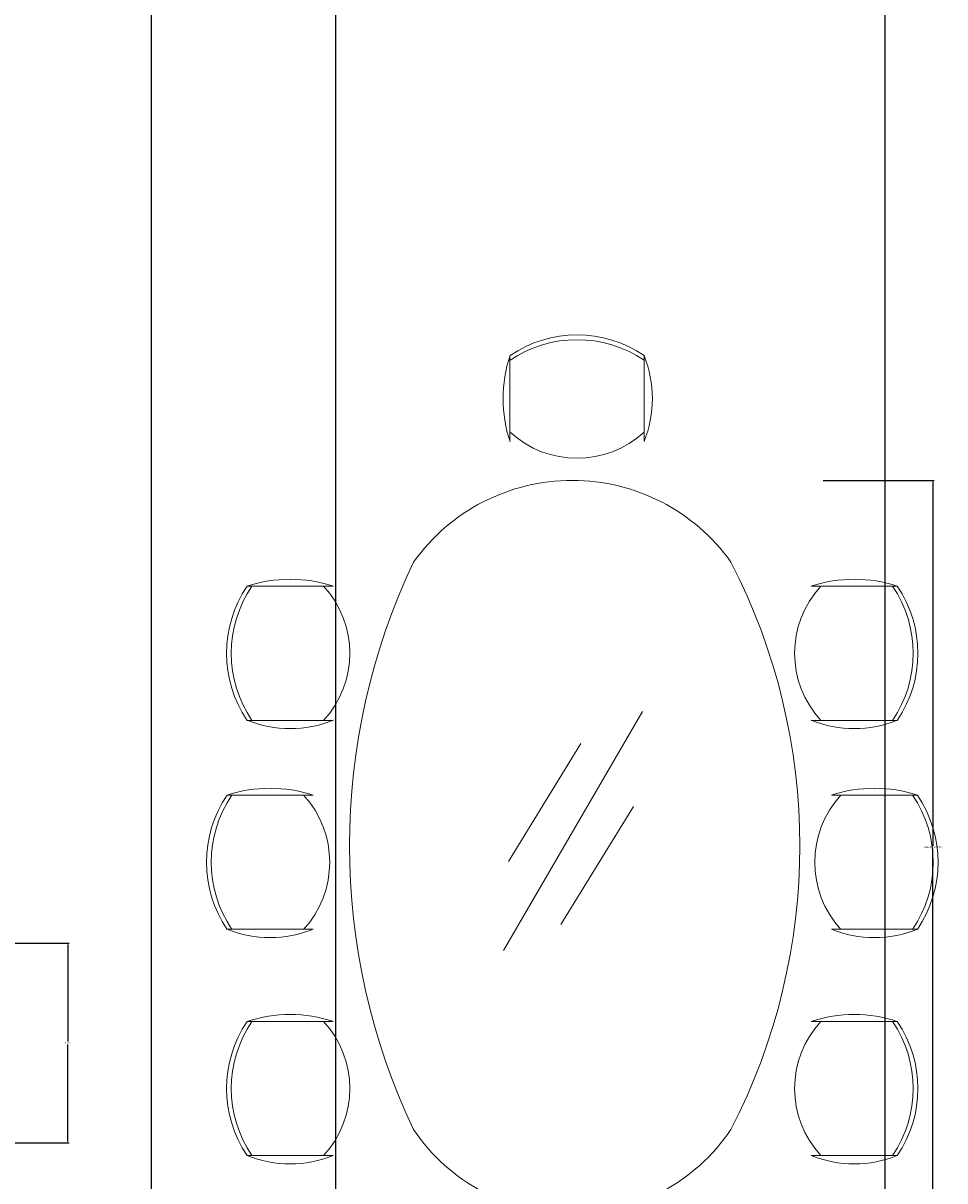
# Model space of a CAD drawing. Units: inches. Extents: x -61 to 1599, y -1316 to 257.
# Tile 125 of 204: x 236 to 356, y -166 to -16. Entities that reach past the tile are written whole.
import ezdxf

# ---------------------------------------------------------------- set-up
doc = ezdxf.new("R2010")
doc.units = ezdxf.units.IN
doc.header["$MEASUREMENT"] = 0
doc.layers.add('A-ANNO-DIMS', color=2, linetype='Continuous', lineweight=18)
doc.layers.add('FURNITURE', color=83, linetype='Continuous', lineweight=18)
doc.styles.get("Standard").update_dxf_attribs({"font": 'arial.ttf'})
doc.dimstyles.get("Standard").update_dxf_attribs({"dimtxt": 0.18, "dimasz": 0.18, "dimexe": 0.18, "dimexo": 0.0625, "dimgap": 0.09, "dimtad": 0, "dimtih": 1, "dimtoh": 1, "dimdec": 0, "dimzin": 0, "dimdsep": 46, "dimlunit": 3, "dimtxsty": 'Standard', "dimcen": 0.09, "dimadec": 0, "dimazin": 0, "dimtfac": 1, "dimtdec": 0, "dimtofl": 0, "dimtmove": 0, "dimatfit": 3, "dimfxl": 1, "dimtolj": 1, "dimtzin": 0, "dimarcsym": 0})

# ---------------------------------------------------------------- blocks, each defined once
blk = doc.blocks.new('DINING-TABLE-OVAL')
for p, q in [((20.06, 34.26), (38.12, 65.35)), ((20.69, 45.86), (30.12, 61.18)), ((27.51, 37.68), (36.94, 53.01))]:
    blk.add_line(p, q)
for centre, radius, start, end in [((28.99, 70.07), 25.36, 35.5172, 144.4828), ((85.79, 47.89), 85.79, 154.5151, 205.4849), ((-21.85, 47.89), 80.45, 332.689, 27.311), ((28.99, 24.89), 24.89, 213.9753, 326.0247)]:
    blk.add_arc(centre, radius, start, end)
blk = doc.blocks.new('DINING-CHAIR')
for p, q in [((0.9, 2.16), (0.9, 13.35)), ((18.35, 2.16), (18.35, 13.35))]:
    blk.add_line(p, q)
for centre, radius, start, end in [((9.63, 0.52), 15.52, 55.8098, 124.1902), ((9.63, -0.1), 15.52, 55.8098, 124.1902), ((17.78, 7.76), 17.78, 161.6455, 198.3545), ((4.51, 7.76), 14.92, 337.9646, 22.0354), ((9.63, 12.87), 12.87, 227.332, 312.668)]:
    blk.add_arc(centre, radius, start, end)
blk = doc.blocks.new('*D666')
at = {"layer": 'A-ANNO-DIMS', "color": 0, "lineweight": -2, "transparency": 16777216}
for p, q in [((340.28, -75.2), (354.71, -75.2)), ((354.53, -75.38), (354.53, -122.73)), ((354.53, -170.45), (354.53, -123.09)), ((340.28, -170.63), (354.71, -170.63))]:
    blk.add_line(p, q, dxfattribs=at)
at = {"layer": 'A-ANNO-DIMS', "color": 0, "transparency": 16777216}
for points in [[(354.5, -75.38), (354.56, -75.38), (354.53, -75.2)], [(354.5, -170.45), (354.56, -170.45), (354.53, -170.63)]]:
    blk.add_solid(points, dxfattribs=at)
at = {"layer": 'DEFPOINTS', "color": 0, "transparency": 16777216}
for p in [(340.22, -75.2), (354.53, -75.2), (340.22, -170.63)]:
    blk.add_point(p, dxfattribs=at)
at = {"layer": 'A-ANNO-DIMS', "color": 0, "transparency": 16777216, "insert": (354.53, -122.91), "char_height": 0.18, "attachment_point": 5}
blk.add_mtext('\\A1;DINING TABLE 95 TYP.', dxfattribs=at)
blk = doc.blocks.new('*D671')
at = {"layer": 'A-ANNO-DIMS', "color": 0, "lineweight": -2, "transparency": 16777216}
for p, q in [((229.44, -135.38), (242.15, -135.38)), ((241.97, -135.56), (241.97, -148.2)), ((241.97, -161.2), (241.97, -148.56)), ((229.44, -161.38), (242.15, -161.38))]:
    blk.add_line(p, q, dxfattribs=at)
at = {"layer": 'A-ANNO-DIMS', "color": 0, "transparency": 16777216}
for points in [[(241.94, -135.56), (242, -135.56), (241.97, -135.38)], [(241.94, -161.2), (242, -161.2), (241.97, -161.38)]]:
    blk.add_solid(points, dxfattribs=at)
at = {"layer": 'DEFPOINTS', "color": 0, "transparency": 16777216}
for p in [(229.37, -135.38), (241.97, -135.38), (229.37, -161.38)]:
    blk.add_point(p, dxfattribs=at)
at = {"layer": 'A-ANNO-DIMS', "color": 0, "transparency": 16777216, "insert": (241.97, -148.38), "char_height": 0.18, "attachment_point": 5}
blk.add_mtext('\\A1;26 TYP.', dxfattribs=at)
blk = doc.blocks.new('*D687')
at = {"layer": 'A-ANNO-DIMS', "color": 0, "lineweight": -2, "transparency": 16777216}
for p, q in [((289.42, 181.68), (-61.08, 181.68)), ((-60.9, 181.5), (-60.9, -528.95)), ((-60.9, -1239.76), (-60.9, -529.32)), ((319.64, -1239.94), (-61.08, -1239.94))]:
    blk.add_line(p, q, dxfattribs=at)
at = {"layer": 'A-ANNO-DIMS', "color": 0, "transparency": 16777216}
for points in [[(-60.93, 181.5), (-60.87, 181.5), (-60.9, 181.68)], [(-60.93, -1239.76), (-60.87, -1239.76), (-60.9, -1239.94)]]:
    blk.add_solid(points, dxfattribs=at)
at = {"layer": 'DEFPOINTS', "color": 0, "transparency": 16777216}
for p in [(289.48, 181.68), (-60.9, -1239.94), (319.7, -1239.94)]:
    blk.add_point(p, dxfattribs=at)
at = {"layer": 'A-ANNO-DIMS', "color": 0, "transparency": 16777216, "insert": (-60.9, -529.13), "char_height": 0.18, "attachment_point": 5}
blk.add_mtext('\\A1;1421.6', dxfattribs=at)
blk = doc.blocks.new('*D701')
at = {"layer": 'A-ANNO-DIMS', "color": 0, "lineweight": -2, "transparency": 16777216}
for p, q in [((215.75, -616.88), (215.75, 257.46)), ((215.93, 257.28), (233.92, 257.28)), ((252.7, 257.28), (234.71, 257.28)), ((252.88, -616.88), (252.88, 257.46))]:
    blk.add_line(p, q, dxfattribs=at)
at = {"layer": 'A-ANNO-DIMS', "color": 0, "transparency": 16777216}
for points in [[(215.93, 257.31), (215.93, 257.25), (215.75, 257.28)], [(252.7, 257.31), (252.7, 257.25), (252.88, 257.28)]]:
    blk.add_solid(points, dxfattribs=at)
at = {"layer": 'DEFPOINTS', "color": 0, "transparency": 16777216}
for p in [(252.88, 257.28), (215.75, -616.94), (252.88, -616.94)]:
    blk.add_point(p, dxfattribs=at)
at = {"layer": 'A-ANNO-DIMS', "color": 0, "transparency": 16777216, "insert": (234.32, 257.28), "char_height": 0.18, "attachment_point": 5}
blk.add_mtext('\\A1;37.13', dxfattribs=at)
blk = doc.blocks.new('*D702')
at = {"layer": 'A-ANNO-DIMS', "color": 0, "lineweight": -2, "transparency": 16777216}
for p, q in [((276.88, -616.88), (276.88, 257.46)), ((277.06, 257.28), (312.21, 257.28)), ((348.14, 257.28), (312.99, 257.28)), ((348.32, -616.88), (348.32, 257.46))]:
    blk.add_line(p, q, dxfattribs=at)
at = {"layer": 'A-ANNO-DIMS', "color": 0, "transparency": 16777216}
for points in [[(277.06, 257.31), (277.06, 257.25), (276.88, 257.28)], [(348.14, 257.31), (348.14, 257.25), (348.32, 257.28)]]:
    blk.add_solid(points, dxfattribs=at)
at = {"layer": 'DEFPOINTS', "color": 0, "transparency": 16777216}
for p in [(348.32, 257.28), (276.88, -616.94), (348.32, -616.94)]:
    blk.add_point(p, dxfattribs=at)
at = {"layer": 'A-ANNO-DIMS', "color": 0, "transparency": 16777216, "insert": (312.6, 257.28), "char_height": 0.18, "attachment_point": 5}
blk.add_mtext('\\A1;71.44', dxfattribs=at)

msp = doc.modelspace()

# ---------------------------------------------------------------- block references
at = {"layer": 'FURNITURE'}
for name, p in [('DINING-CHAIR', (298.622, -72.324)), ('DINING-TABLE-OVAL', (278.634, -170.626))]:
    msp.add_blockref(name, p, dxfattribs=at)
at = {"layer": 'FURNITURE', "extrusion": (0, 0, -1), "zscale": -1}
for p, rotation in [((-278.681, -88.0629), 269.9999999999997), ((-276.0669, -115.2445), 269.9999999999993), ((-278.681, -144.6698), 270.0000000000002)]:
    msp.add_blockref('DINING-CHAIR', p, dxfattribs=dict(at, rotation=rotation))
at = {"layer": 'FURNITURE'}
for p, rotation in [((336.562, -88.0629), 269.9999999999997), ((339.1761, -115.2445), 269.9999999999999), ((336.562, -144.6698), 269.9999999999998)]:
    msp.add_blockref('DINING-CHAIR', p, dxfattribs=dict(at, rotation=rotation))

# ---------------------------------------------------------------- dimensions: what is measured, and where the dimension line sits
at = {"layer": 'A-ANNO-DIMS'}
for base, p1, p2, picture, middle in [((252.8825, 257.2771), (215.7521, -616.9446), (252.8825, -616.9446), '*D701', (234.3173, 257.2771)), ((348.3201, 257.2771), (276.8825, -616.9446), (348.3201, -616.9446), '*D702', (312.6013, 257.2771))]:
    dim = msp.add_linear_dim(base=base, p1=p1, p2=p2, dimstyle='Standard', override={"dimdec": 2, "dimlfac": 1, "dimrnd": 0, "dimzin": 0, "dimdsep": 46, "dimlunit": 2}, dxfattribs=at)
    dim.commit()
    dim.dimension.update_dxf_attribs({"geometry": picture, "text_midpoint": middle})
dim = msp.add_linear_dim(base=(-60.8972, -1239.9446), p1=(289.4807, 181.6771), p2=(319.7028, -1239.9446), angle=90, dimstyle='Standard', override={"dimdec": 1, "dimlfac": 1, "dimrnd": 0, "dimzin": 0, "dimdsep": 46, "dimlunit": 2}, dxfattribs=at)
dim.commit()
dim.dimension.update_dxf_attribs({"geometry": '*D687', "text_midpoint": (-60.8972, -529.1337)})
for base, p1, p2, text, picture, middle in [((354.533, -75.1959), (340.2185, -170.6256), (340.2185, -75.1959), 'DINING TABLE <> TYP.', '*D666', (354.533, -122.9108)), ((241.9746, -135.3792), (229.3746, -161.3792), (229.3746, -135.3792), '<> TYP.', '*D671', (241.9746, -148.3792))]:
    dim = msp.add_linear_dim(base=base, p1=p1, p2=p2, angle=90, text=text, dimstyle='Standard', override={"dimdec": 0, "dimlfac": 1, "dimrnd": 0, "dimzin": 0, "dimdsep": 46, "dimlunit": 2}, dxfattribs=at)
    dim.commit()
    dim.dimension.update_dxf_attribs({"geometry": picture, "text_midpoint": middle})

doc.saveas('drawing.dxf')
